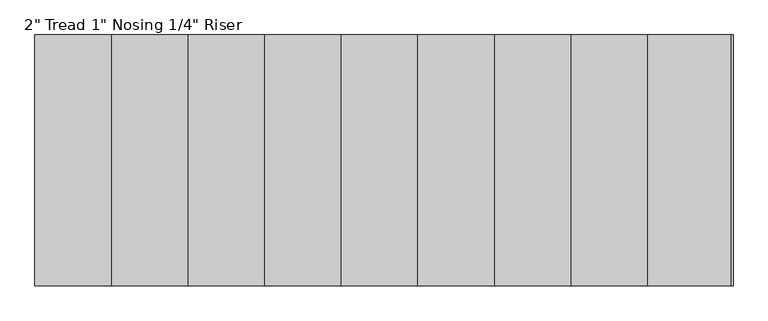
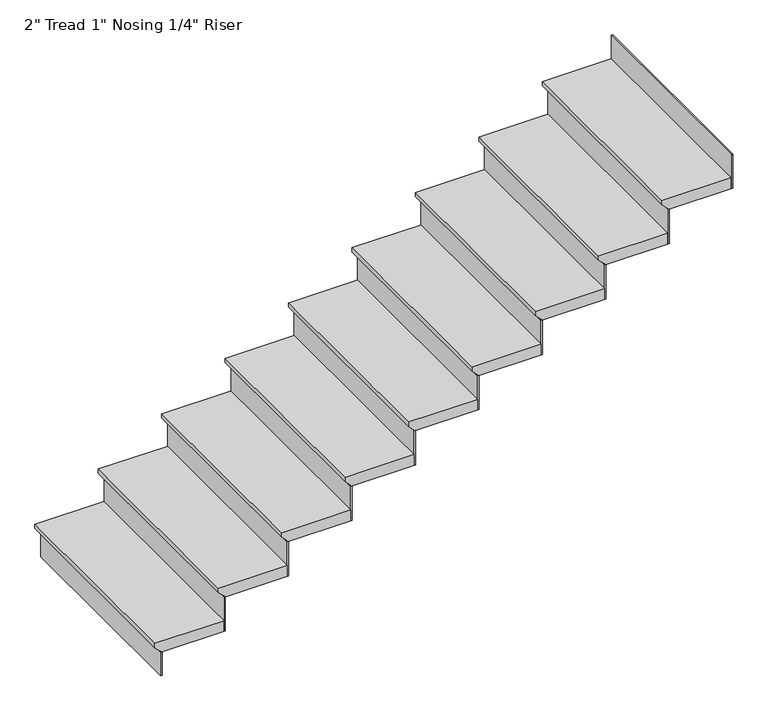
"""IFC4 building model written with IfcOpenShell, lengths in millimetres: stair flight geometry."""

from ifc_helpers import new_model, si_unit, origin, place, context, project, spatial, faceted_brep, source, transform, mapped, element, save


def stair_flight_4ab4d81b(model_context):
    return source(origin(), model_context, "Body", "Brep", [
        faceted_brep([(-1591.1154463, -4737.3544725, 6541.77), (-1591.1154463, -4737.3544725, 6560.82), (-1591.1154463, -3822.9544725, 6560.82), (-1591.1154463, -3822.9544725, 6541.77), (-1565.7154463, -4737.3544725, 6516.37), (-1565.7154463, -3822.9544725, 6516.37), (-1286.3154463, -4737.3544725, 6560.82), (-1286.3154463, -3822.9544725, 6560.82), (-1565.7154463, -3822.9544725, 6510.02), (-1286.3154463, -3822.9544725, 6510.02), (-1286.3154463, -4737.3544725, 6510.02), (-1565.7154463, -4737.3544725, 6510.02)], [[[0, 1, 2, 3]], [[4, 0, 3, 5]], [[2, 1, 6, 7]], [[8, 9, 10, 11]], [[2, 7, 9, 8, 5, 3]], [[8, 11, 4, 5]], [[6, 1, 0, 4, 11, 10]], [[7, 6, 10, 9]]]),
        faceted_brep([(-1565.7154463, -4737.3544725, 6510.02), (-1565.7154463, -4737.3544725, 6400.8), (-1559.3654463, -4737.3544725, 6400.8), (-1559.3654463, -4737.3544725, 6510.02), (-1565.7154463, -3822.9544725, 6510.02), (-1559.3654463, -3822.9544725, 6510.02), (-1559.3654463, -3822.9544725, 6400.8), (-1565.7154463, -3822.9544725, 6400.8)], [[[0, 1, 2, 3]], [[4, 5, 6, 7]], [[1, 0, 4, 7]], [[2, 1, 7, 6]], [[3, 2, 6, 5]], [[0, 3, 5, 4]]]),
        faceted_brep([(-1286.3154463, -4737.3544725, 6670.04), (-1286.3154463, -4737.3544725, 6510.02), (-1279.9654463, -4737.3544725, 6510.02), (-1279.9654463, -4737.3544725, 6670.04), (-1286.3154463, -3822.9544725, 6670.04), (-1279.9654463, -3822.9544725, 6670.04), (-1279.9654463, -3822.9544725, 6510.02), (-1286.3154463, -3822.9544725, 6510.02)], [[[0, 1, 2, 3]], [[4, 5, 6, 7]], [[1, 0, 4, 7]], [[2, 1, 7, 6]], [[3, 2, 6, 5]], [[0, 3, 5, 4]]]),
        faceted_brep([(-1311.7154463, -3822.9544725, 6720.84), (-1311.7154463, -4737.3544725, 6720.84), (-1006.9154463, -4737.3544725, 6720.84), (-1006.9154463, -3822.9544725, 6720.84), (-1286.3154463, -3822.9544725, 6670.04), (-1006.9154463, -3822.9544725, 6670.04), (-1006.9154463, -4737.3544725, 6670.04), (-1286.3154463, -4737.3544725, 6670.04), (-1286.3154463, -3822.9544725, 6676.39), (-1311.7154463, -3822.9544725, 6701.79), (-1286.3154463, -4737.3544725, 6676.39), (-1311.7154463, -4737.3544725, 6701.79)], [[[0, 1, 2, 3]], [[4, 5, 6, 7]], [[0, 3, 5, 4, 8, 9]], [[4, 7, 10, 8]], [[2, 1, 11, 10, 7, 6]], [[3, 2, 6, 5]], [[11, 1, 0, 9]], [[10, 11, 9, 8]]]),
        faceted_brep([(-1006.9154463, -4737.3544725, 6830.06), (-1006.9154463, -4737.3544725, 6670.04), (-1000.5654463, -4737.3544725, 6670.04), (-1000.5654463, -4737.3544725, 6830.06), (-1006.9154463, -3822.9544725, 6830.06), (-1000.5654463, -3822.9544725, 6830.06), (-1000.5654463, -3822.9544725, 6670.04), (-1006.9154463, -3822.9544725, 6670.04)], [[[0, 1, 2, 3]], [[4, 5, 6, 7]], [[1, 0, 4, 7]], [[2, 1, 7, 6]], [[3, 2, 6, 5]], [[0, 3, 5, 4]]]),
        faceted_brep([(-1032.3154463, -3822.9544725, 6880.86), (-1032.3154463, -4737.3544725, 6880.86), (-727.5154463, -4737.3544725, 6880.86), (-727.5154463, -3822.9544725, 6880.86), (-1006.9154463, -3822.9544725, 6830.06), (-727.5154463, -3822.9544725, 6830.06), (-727.5154463, -4737.3544725, 6830.06), (-1006.9154463, -4737.3544725, 6830.06), (-1006.9154463, -3822.9544725, 6836.41), (-1032.3154463, -3822.9544725, 6861.81), (-1006.9154463, -4737.3544725, 6836.41), (-1032.3154463, -4737.3544725, 6861.81)], [[[0, 1, 2, 3]], [[4, 5, 6, 7]], [[0, 3, 5, 4, 8, 9]], [[4, 7, 10, 8]], [[2, 1, 11, 10, 7, 6]], [[3, 2, 6, 5]], [[11, 1, 0, 9]], [[10, 11, 9, 8]]]),
        faceted_brep([(-727.5154463, -4737.3544725, 6990.08), (-727.5154463, -4737.3544725, 6830.06), (-721.1654463, -4737.3544725, 6830.06), (-721.1654463, -4737.3544725, 6990.08), (-727.5154463, -3822.9544725, 6990.08), (-721.1654463, -3822.9544725, 6990.08), (-721.1654463, -3822.9544725, 6830.06), (-727.5154463, -3822.9544725, 6830.06)], [[[0, 1, 2, 3]], [[4, 5, 6, 7]], [[1, 0, 4, 7]], [[2, 1, 7, 6]], [[3, 2, 6, 5]], [[0, 3, 5, 4]]]),
        faceted_brep([(-752.9154463, -3822.9544725, 7040.88), (-752.9154463, -4737.3544725, 7040.88), (-448.1154463, -4737.3544725, 7040.88), (-448.1154463, -3822.9544725, 7040.88), (-727.5154463, -3822.9544725, 6990.08), (-448.1154463, -3822.9544725, 6990.08), (-448.1154463, -4737.3544725, 6990.08), (-727.5154463, -4737.3544725, 6990.08), (-727.5154463, -3822.9544725, 6996.43), (-752.9154463, -3822.9544725, 7021.83), (-727.5154463, -4737.3544725, 6996.43), (-752.9154463, -4737.3544725, 7021.83)], [[[0, 1, 2, 3]], [[4, 5, 6, 7]], [[0, 3, 5, 4, 8, 9]], [[4, 7, 10, 8]], [[2, 1, 11, 10, 7, 6]], [[3, 2, 6, 5]], [[11, 1, 0, 9]], [[10, 11, 9, 8]]]),
        faceted_brep([(-448.1154463, -4737.3544725, 7150.1), (-448.1154463, -4737.3544725, 6990.08), (-441.7654463, -4737.3544725, 6990.08), (-441.7654463, -4737.3544725, 7150.1), (-448.1154463, -3822.9544725, 7150.1), (-441.7654463, -3822.9544725, 7150.1), (-441.7654463, -3822.9544725, 6990.08), (-448.1154463, -3822.9544725, 6990.08)], [[[0, 1, 2, 3]], [[4, 5, 6, 7]], [[1, 0, 4, 7]], [[2, 1, 7, 6]], [[3, 2, 6, 5]], [[0, 3, 5, 4]]]),
        faceted_brep([(-473.5154463, -3822.9544725, 7200.9), (-473.5154463, -4737.3544725, 7200.9), (-168.7154463, -4737.3544725, 7200.9), (-168.7154463, -3822.9544725, 7200.9), (-448.1154463, -3822.9544725, 7150.1), (-168.7154463, -3822.9544725, 7150.1), (-168.7154463, -4737.3544725, 7150.1), (-448.1154463, -4737.3544725, 7150.1), (-448.1154463, -3822.9544725, 7156.45), (-473.5154463, -3822.9544725, 7181.85), (-448.1154463, -4737.3544725, 7156.45), (-473.5154463, -4737.3544725, 7181.85)], [[[0, 1, 2, 3]], [[4, 5, 6, 7]], [[0, 3, 5, 4, 8, 9]], [[4, 7, 10, 8]], [[2, 1, 11, 10, 7, 6]], [[3, 2, 6, 5]], [[11, 1, 0, 9]], [[10, 11, 9, 8]]]),
        faceted_brep([(-168.7154463, -4737.3544725, 7310.12), (-168.7154463, -4737.3544725, 7150.1), (-162.3654463, -4737.3544725, 7150.1), (-162.3654463, -4737.3544725, 7310.12), (-168.7154463, -3822.9544725, 7310.12), (-162.3654463, -3822.9544725, 7310.12), (-162.3654463, -3822.9544725, 7150.1), (-168.7154463, -3822.9544725, 7150.1)], [[[0, 1, 2, 3]], [[4, 5, 6, 7]], [[1, 0, 4, 7]], [[2, 1, 7, 6]], [[3, 2, 6, 5]], [[0, 3, 5, 4]]]),
        faceted_brep([(-194.1154463, -3822.9544725, 7360.92), (-194.1154463, -4737.3544725, 7360.92), (110.6845537, -4737.3544725, 7360.92), (110.6845537, -3822.9544725, 7360.92), (-168.7154463, -3822.9544725, 7310.12), (110.6845537, -3822.9544725, 7310.12), (110.6845537, -4737.3544725, 7310.12), (-168.7154463, -4737.3544725, 7310.12), (-168.7154463, -3822.9544725, 7316.47), (-194.1154463, -3822.9544725, 7341.87), (-168.7154463, -4737.3544725, 7316.47), (-194.1154463, -4737.3544725, 7341.87)], [[[0, 1, 2, 3]], [[4, 5, 6, 7]], [[0, 3, 5, 4, 8, 9]], [[4, 7, 10, 8]], [[2, 1, 11, 10, 7, 6]], [[3, 2, 6, 5]], [[11, 1, 0, 9]], [[10, 11, 9, 8]]]),
        faceted_brep([(110.6845537, -4737.3544725, 7470.14), (110.6845537, -4737.3544725, 7310.12), (117.0345537, -4737.3544725, 7310.12), (117.0345537, -4737.3544725, 7470.14), (110.6845537, -3822.9544725, 7470.14), (117.0345537, -3822.9544725, 7470.14), (117.0345537, -3822.9544725, 7310.12), (110.6845537, -3822.9544725, 7310.12)], [[[0, 1, 2, 3]], [[4, 5, 6, 7]], [[1, 0, 4, 7]], [[2, 1, 7, 6]], [[3, 2, 6, 5]], [[0, 3, 5, 4]]]),
        faceted_brep([(85.2845537, -3822.9544725, 7520.94), (85.2845537, -4737.3544725, 7520.94), (390.0845537, -4737.3544725, 7520.94), (390.0845537, -3822.9544725, 7520.94), (110.6845537, -3822.9544725, 7470.14), (390.0845537, -3822.9544725, 7470.14), (390.0845537, -4737.3544725, 7470.14), (110.6845537, -4737.3544725, 7470.14), (110.6845537, -3822.9544725, 7476.49), (85.2845537, -3822.9544725, 7501.89), (110.6845537, -4737.3544725, 7476.49), (85.2845537, -4737.3544725, 7501.89)], [[[0, 1, 2, 3]], [[4, 5, 6, 7]], [[0, 3, 5, 4, 8, 9]], [[4, 7, 10, 8]], [[2, 1, 11, 10, 7, 6]], [[3, 2, 6, 5]], [[11, 1, 0, 9]], [[10, 11, 9, 8]]]),
        faceted_brep([(390.0845537, -4737.3544725, 7630.16), (390.0845537, -4737.3544725, 7470.14), (396.4345537, -4737.3544725, 7470.14), (396.4345537, -4737.3544725, 7630.16), (390.0845537, -3822.9544725, 7630.16), (396.4345537, -3822.9544725, 7630.16), (396.4345537, -3822.9544725, 7470.14), (390.0845537, -3822.9544725, 7470.14)], [[[0, 1, 2, 3]], [[4, 5, 6, 7]], [[1, 0, 4, 7]], [[2, 1, 7, 6]], [[3, 2, 6, 5]], [[0, 3, 5, 4]]]),
        faceted_brep([(364.6845537, -3822.9544725, 7680.96), (364.6845537, -4737.3544725, 7680.96), (669.4845537, -4737.3544725, 7680.96), (669.4845537, -3822.9544725, 7680.96), (390.0845537, -3822.9544725, 7630.16), (669.4845537, -3822.9544725, 7630.16), (669.4845537, -4737.3544725, 7630.16), (390.0845537, -4737.3544725, 7630.16), (390.0845537, -3822.9544725, 7636.51), (364.6845537, -3822.9544725, 7661.91), (390.0845537, -4737.3544725, 7636.51), (364.6845537, -4737.3544725, 7661.91)], [[[0, 1, 2, 3]], [[4, 5, 6, 7]], [[0, 3, 5, 4, 8, 9]], [[4, 7, 10, 8]], [[2, 1, 11, 10, 7, 6]], [[3, 2, 6, 5]], [[11, 1, 0, 9]], [[10, 11, 9, 8]]]),
        faceted_brep([(948.8845537, -4737.3544725, 7950.2), (948.8845537, -4737.3544725, 7790.18), (955.2345537, -4737.3544725, 7790.18), (955.2345537, -4737.3544725, 7950.2), (948.8845537, -3822.9544725, 7950.2), (955.2345537, -3822.9544725, 7950.2), (955.2345537, -3822.9544725, 7790.18), (948.8845537, -3822.9544725, 7790.18)], [[[0, 1, 2, 3]], [[4, 5, 6, 7]], [[1, 0, 4, 7]], [[2, 1, 7, 6]], [[3, 2, 6, 5]], [[0, 3, 5, 4]]]),
        faceted_brep([(669.4845537, -4737.3544725, 7790.18), (669.4845537, -4737.3544725, 7630.16), (675.8345537, -4737.3544725, 7630.16), (675.8345537, -4737.3544725, 7790.18), (669.4845537, -3822.9544725, 7790.18), (675.8345537, -3822.9544725, 7790.18), (675.8345537, -3822.9544725, 7630.16), (669.4845537, -3822.9544725, 7630.16)], [[[0, 1, 2, 3]], [[4, 5, 6, 7]], [[1, 0, 4, 7]], [[2, 1, 7, 6]], [[3, 2, 6, 5]], [[0, 3, 5, 4]]]),
        faceted_brep([(948.8845537, -3822.9544725, 7840.98), (923.4845537, -3822.9544725, 7840.98), (644.0845537, -3822.9544725, 7840.98), (644.0845537, -4737.3544725, 7840.98), (948.8845537, -4737.3544725, 7840.98), (923.4845537, -3822.9544725, 7790.18), (948.8845537, -3822.9544725, 7790.18), (948.8845537, -4737.3544725, 7790.18), (669.4845537, -4737.3544725, 7790.18), (669.4845537, -3822.9544725, 7790.18), (669.4845537, -3822.9544725, 7796.53), (644.0845537, -3822.9544725, 7821.93), (669.4845537, -4737.3544725, 7796.53), (644.0845537, -4737.3544725, 7821.93)], [[[0, 1, 2, 3, 4]], [[5, 6, 7, 8, 9]], [[1, 0, 6, 5]], [[2, 1, 5, 9, 10, 11]], [[9, 8, 12, 10]], [[4, 3, 13, 12, 8, 7]], [[0, 4, 7, 6]], [[13, 3, 2, 11]], [[12, 13, 11, 10]]]),
    ])


if __name__ == "__main__":
    model = new_model("IFC4")
    model_context = context("Model", 3, world=origin())
    ifc_project = project(units=[si_unit("LENGTHUNIT", "METRE", prefix="MILLI")], contexts=[model_context])
    site = spatial("IfcSite", under=ifc_project)
    building = spatial("IfcBuilding", under=site)
    placement = place(None, origin())
    stair_flight_shape = stair_flight_4ab4d81b(model_context)
    element("IfcStairFlight", 1, ObjectType="2\" Tread 1\" Nosing 1/4\" Riser", at=placement, inside=building, context=model_context, shape_type="MappedRepresentation", body=[
        mapped(stair_flight_shape, transform((0.0, 0.0, 0.0), x_axis=(1.0, 0.0, 0.0), y_axis=(0.0, 1.0, 0.0), z_axis=(0.0, 0.0, 1.0))),
    ])
    save(model, "model.ifc")
